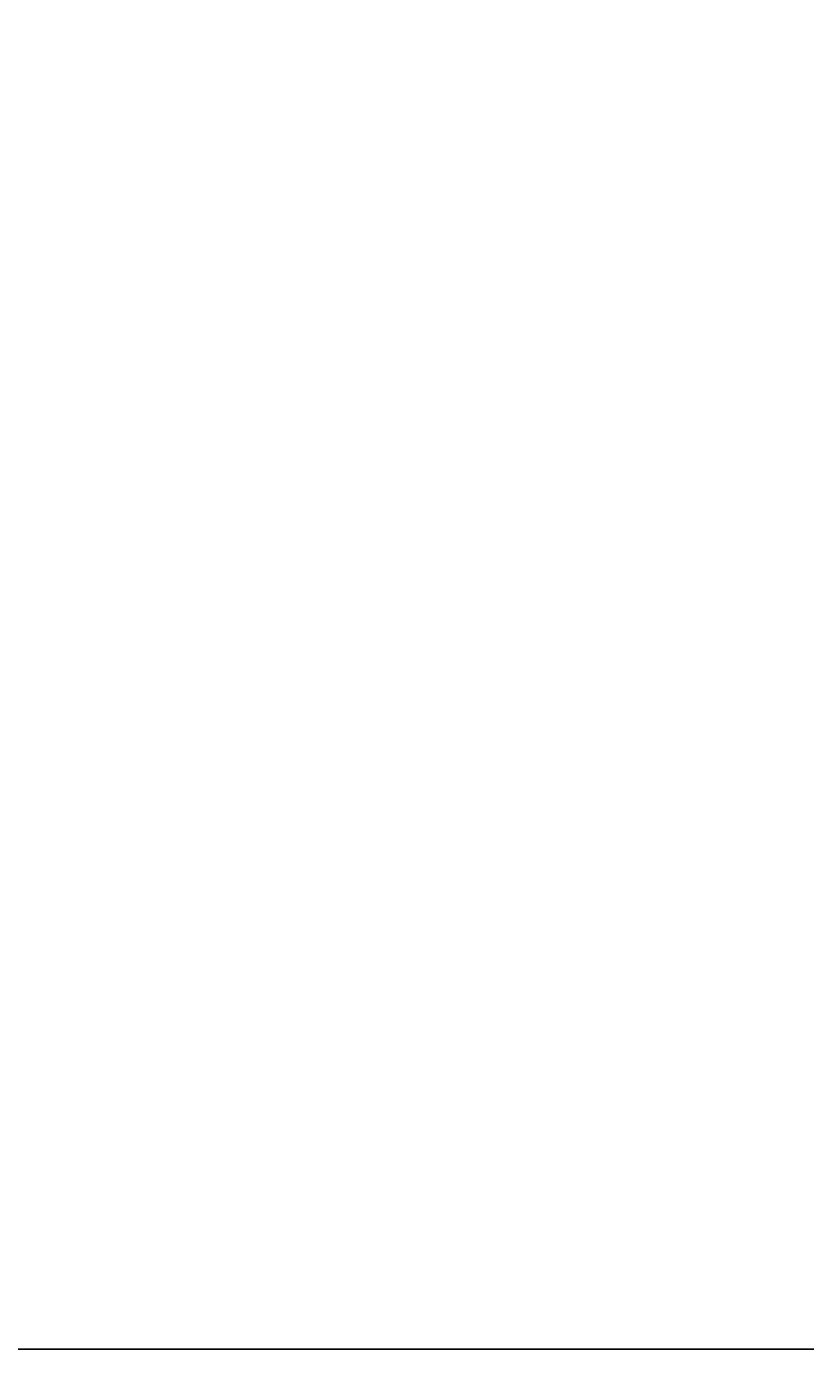
# Model space of a CAD drawing. Units: feet. Extents: x 105 to 1094, y -88 to 588.
# Tile 49 of 59: x 575 to 600, y 470 to 513. Entities that reach past the tile are written whole.
import ezdxf

# ---------------------------------------------------------------- set-up
doc = ezdxf.new("R2010")
doc.units = ezdxf.units.FT
doc.header["$MEASUREMENT"] = 0
doc.layers.add('A-ANNO-DIMS', color=2, linetype='Continuous', lineweight=18)
doc.styles.get("Standard").update_dxf_attribs({"font": 'arial.ttf'})
doc.dimstyles.get("Standard").update_dxf_attribs({"dimtxt": 0.18, "dimasz": 0.18, "dimexe": 0.18, "dimexo": 0.0625, "dimgap": 0.09, "dimtad": 0, "dimtih": 1, "dimtoh": 1, "dimdec": 4, "dimzin": 0, "dimdsep": 46, "dimtxsty": 'Standard', "dimcen": 0.09, "dimadec": 0, "dimazin": 0, "dimtfac": 1, "dimtdec": 4, "dimtofl": 0, "dimtmove": 0, "dimatfit": 3, "dimfxl": 1, "dimtolj": 1, "dimtzin": 0, "dimarcsym": 0})

# ---------------------------------------------------------------- blocks, each defined once
blk = doc.blocks.new('*D21')
at = {"layer": 'A-ANNO-DIMS', "color": 0, "lineweight": -2, "transparency": 16777216}
for p, q in [((849.626, 543.081), (105.458, 543.081)), ((105.638, 542.901), (105.638, 250.263)), ((105.638, -42.739), (105.638, 249.899)), ((849.626, -42.919), (105.458, -42.919))]:
    blk.add_line(p, q, dxfattribs=at)
at = {"layer": 'A-ANNO-DIMS', "color": 0, "transparency": 16777216}
for points in [[(105.608, 542.901), (105.668, 542.901), (105.638, 543.081)], [(105.608, -42.739), (105.668, -42.739), (105.638, -42.919)]]:
    blk.add_solid(points, dxfattribs=at)
at = {"layer": 'Defpoints', "color": 0, "transparency": 16777216}
for p in [(105.638, 543.081), (849.688, 543.081), (849.688, -42.919)]:
    blk.add_point(p, dxfattribs=at)
at = {"layer": 'A-ANNO-DIMS', "color": 0, "transparency": 16777216, "insert": (105.638, 250.081), "char_height": 0.18, "attachment_point": 5}
blk.add_mtext('\\A1;586', dxfattribs=at)
blk = doc.blocks.new('*D26')
at = {"layer": 'A-ANNO-DIMS', "color": 0, "lineweight": -2, "transparency": 16777216}
for p, q in [((552.688, 471.144), (552.688, 588.311)), ((552.868, 588.131), (599.47, 588.131)), ((646.508, 588.131), (599.907, 588.131)), ((646.688, 471.144), (646.688, 588.311))]:
    blk.add_line(p, q, dxfattribs=at)
at = {"layer": 'A-ANNO-DIMS', "color": 0, "transparency": 16777216}
for points in [[(552.868, 588.161), (552.868, 588.101), (552.688, 588.131)], [(646.508, 588.161), (646.508, 588.101), (646.688, 588.131)]]:
    blk.add_solid(points, dxfattribs=at)
at = {"layer": 'Defpoints', "color": 0, "transparency": 16777216}
for p in [(646.688, 588.131), (552.688, 471.081), (646.688, 471.081)]:
    blk.add_point(p, dxfattribs=at)
at = {"layer": 'A-ANNO-DIMS', "color": 0, "transparency": 16777216, "insert": (599.688, 588.131), "char_height": 0.18, "attachment_point": 5}
blk.add_mtext('\\A1;94', dxfattribs=at)
blk = doc.blocks.new('*D31')
at = {"layer": 'A-ANNO-DIMS', "color": 0, "lineweight": -2, "transparency": 16777216}
for p, q in [((438.751, 527.081), (1093.918, 527.081)), ((1093.738, 526.901), (1093.738, 499.263)), ((1093.738, 471.261), (1093.738, 498.899)), ((438.751, 471.081), (1093.918, 471.081))]:
    blk.add_line(p, q, dxfattribs=at)
at = {"layer": 'A-ANNO-DIMS', "color": 0, "transparency": 16777216}
for points in [[(1093.708, 526.901), (1093.768, 526.901), (1093.738, 527.081)], [(1093.708, 471.261), (1093.768, 471.261), (1093.738, 471.081)]]:
    blk.add_solid(points, dxfattribs=at)
at = {"layer": 'Defpoints', "color": 0, "transparency": 16777216}
for p in [(438.688, 527.081), (1093.738, 527.081), (438.688, 471.081)]:
    blk.add_point(p, dxfattribs=at)
at = {"layer": 'A-ANNO-DIMS', "color": 0, "transparency": 16777216, "insert": (1093.738, 499.081), "char_height": 0.18, "attachment_point": 5}
blk.add_mtext('\\A1;56', dxfattribs=at)
blk = doc.blocks.new('*D32')
at = {"layer": 'A-ANNO-DIMS', "color": 0, "lineweight": -2, "transparency": 16777216}
for p, q in [((646.626, 471.081), (105.458, 471.081)), ((105.638, 470.901), (105.638, 456.263)), ((105.638, 441.261), (105.638, 455.899)), ((646.626, 441.081), (105.458, 441.081))]:
    blk.add_line(p, q, dxfattribs=at)
at = {"layer": 'A-ANNO-DIMS', "color": 0, "transparency": 16777216}
for points in [[(105.608, 470.901), (105.668, 470.901), (105.638, 471.081)], [(105.608, 441.261), (105.668, 441.261), (105.638, 441.081)]]:
    blk.add_solid(points, dxfattribs=at)
at = {"layer": 'Defpoints', "color": 0, "transparency": 16777216}
for p in [(105.638, 471.081), (646.688, 471.081), (646.688, 441.081)]:
    blk.add_point(p, dxfattribs=at)
at = {"layer": 'A-ANNO-DIMS', "color": 0, "transparency": 16777216, "insert": (105.638, 456.081), "char_height": 0.18, "attachment_point": 5}
blk.add_mtext('\\A1;30', dxfattribs=at)
blk = doc.blocks.new('*D48')
at = {"layer": 'A-ANNO-DIMS', "color": 0, "lineweight": -2, "transparency": 16777216}
for p, q in [((573.483, 441.144), (573.483, 588.311)), ((573.663, 588.131), (603.263, 588.131)), ((633.303, 588.131), (603.702, 588.131)), ((633.483, 441.144), (633.483, 588.311))]:
    blk.add_line(p, q, dxfattribs=at)
at = {"layer": 'A-ANNO-DIMS', "color": 0, "transparency": 16777216}
for points in [[(573.663, 588.161), (573.663, 588.101), (573.483, 588.131)], [(633.303, 588.161), (633.303, 588.101), (633.483, 588.131)]]:
    blk.add_solid(points, dxfattribs=at)
at = {"layer": 'Defpoints', "color": 0, "transparency": 16777216}
for p in [(633.483, 588.131), (573.483, 441.081), (633.483, 441.081)]:
    blk.add_point(p, dxfattribs=at)
at = {"layer": 'A-ANNO-DIMS', "color": 0, "transparency": 16777216, "insert": (603.483, 588.131), "char_height": 0.18, "attachment_point": 5}
blk.add_mtext('\\A1;60', dxfattribs=at)

msp = doc.modelspace()

# ---------------------------------------------------------------- dimensions: what is measured, and where the dimension line sits
at = {"layer": 'A-ANNO-DIMS'}
for base, p1, p2, picture, middle in [((646.6883, 588.1312), (552.6883, 471.0812), (646.6883, 471.0812), '*D26', (599.6883, 588.1312)), ((633.4826, 588.1312), (573.4826, 441.0812), (633.4826, 441.0812), '*D48', (603.4826, 588.1312))]:
    dim = msp.add_linear_dim(base=base, p1=p1, p2=p2, dimstyle='Standard', override={"dimdec": 0, "dimlfac": 1, "dimrnd": 0, "dimzin": 0, "dimdsep": 46, "dimlunit": 2}, dxfattribs=at)
    dim.commit()
    dim.dimension.update_dxf_attribs({"geometry": picture, "text_midpoint": middle})
for base, p1, p2, picture, middle in [((105.6383, 543.0812), (849.6883, -42.9188), (849.6883, 543.0812), '*D21', (105.6383, 250.0812)), ((1093.7383, 527.0812), (438.6883, 471.0812), (438.6883, 527.0812), '*D31', (1093.7383, 499.0812)), ((105.6383, 471.0812), (646.6883, 441.0812), (646.6883, 471.0812), '*D32', (105.6383, 456.0812))]:
    dim = msp.add_linear_dim(base=base, p1=p1, p2=p2, angle=90, dimstyle='Standard', override={"dimdec": 0, "dimlfac": 1, "dimrnd": 0, "dimzin": 0, "dimdsep": 46, "dimlunit": 2}, dxfattribs=at)
    dim.commit()
    dim.dimension.update_dxf_attribs({"geometry": picture, "text_midpoint": middle})

doc.saveas('drawing.dxf')
